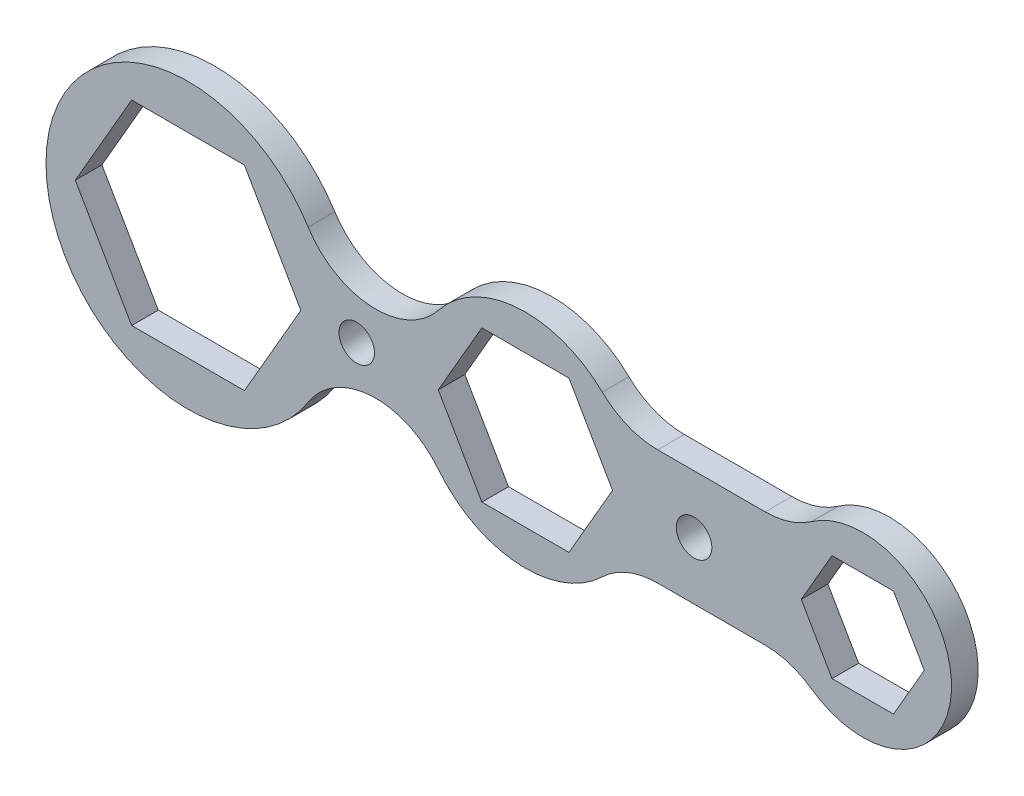
ISO-10303-21;
HEADER;
FILE_DESCRIPTION(('STEP AP214'),'2;1');
FILE_NAME('part.step','',(''),(''),'','','');
FILE_SCHEMA(('AUTOMOTIVE_DESIGN { 1 0 10303 214 1 1 1 1 }'));
ENDSEC;
DATA;
#1=APPLICATION_CONTEXT('core data for automotive mechanical design processes');
#2=APPLICATION_PROTOCOL_DEFINITION('international standard','automotive_design',2000,#1);
#3=PRODUCT_CONTEXT('',#1,'mechanical');
#4=PRODUCT('Part','Part','',(#3));
#5=PRODUCT_RELATED_PRODUCT_CATEGORY('part','',(#4));
#6=PRODUCT_DEFINITION_FORMATION('','',#4);
#7=PRODUCT_DEFINITION_CONTEXT('part definition',#1,'design');
#8=PRODUCT_DEFINITION('design','',#6,#7);
#9=PRODUCT_DEFINITION_SHAPE('','',#8);
#10=(LENGTH_UNIT() NAMED_UNIT(*) SI_UNIT(.MILLI.,.METRE.));
#11=(NAMED_UNIT(*) PLANE_ANGLE_UNIT() SI_UNIT($,.RADIAN.));
#12=(NAMED_UNIT(*) SI_UNIT($,.STERADIAN.) SOLID_ANGLE_UNIT());
#13=UNCERTAINTY_MEASURE_WITH_UNIT(LENGTH_MEASURE(1.E-05),#10,'distance_accuracy_value','');
#14=(GEOMETRIC_REPRESENTATION_CONTEXT(3) GLOBAL_UNCERTAINTY_ASSIGNED_CONTEXT((#13)) GLOBAL_UNIT_ASSIGNED_CONTEXT((#10,
#11,#12)) REPRESENTATION_CONTEXT('',''));
#15=CARTESIAN_POINT('',(0.,0.,0.));
#16=DIRECTION('',(0.,0.,1.));
#17=DIRECTION('',(1.,0.,0.));
#18=AXIS2_PLACEMENT_3D('',#15,#16,#17);
#19=CARTESIAN_POINT('',(76.,0.,6.));
#20=DIRECTION('',(0.,0.,-1.));
#21=DIRECTION('',(-1.,0.,0.));
#22=AXIS2_PLACEMENT_3D('',#19,#20,#21);
#23=CYLINDRICAL_SURFACE('',#22,25.);
#24=CARTESIAN_POINT('',(76.,0.,0.));
#25=DIRECTION('',(0.,0.,1.));
#26=DIRECTION('',(1.,0.,0.));
#27=AXIS2_PLACEMENT_3D('',#24,#25,#26);
#28=CIRCLE('',#27,25.);
#29=CARTESIAN_POINT('',(93.3251911927341,18.0232558139535,0.));
#30=VERTEX_POINT('',#29);
#31=CARTESIAN_POINT('',(56.3970318237454,15.5152711442872,0.));
#32=VERTEX_POINT('',#31);
#33=EDGE_CURVE('E290',#30,#32,#28,.T.);
#34=ORIENTED_EDGE('',*,*,#33,.T.);
#35=DIRECTION('',(0.,0.,-1.));
#36=VECTOR('',#35,1.);
#37=CARTESIAN_POINT('',(56.3970318237454,15.5152711442872,6.));
#38=LINE('',#37,#36);
#39=CARTESIAN_POINT('',(56.3970318237454,15.5152711442872,6.));
#40=VERTEX_POINT('',#39);
#41=EDGE_CURVE('E11',#40,#32,#38,.T.);
#42=ORIENTED_EDGE('',*,*,#41,.F.);
#43=CARTESIAN_POINT('',(76.,0.,6.));
#44=DIRECTION('',(0.,0.,1.));
#45=DIRECTION('',(1.,0.,0.));
#46=AXIS2_PLACEMENT_3D('',#43,#44,#45);
#47=CIRCLE('',#46,25.);
#48=CARTESIAN_POINT('',(93.3251911927341,18.0232558139535,6.));
#49=VERTEX_POINT('',#48);
#50=EDGE_CURVE('E386',#49,#40,#47,.T.);
#51=ORIENTED_EDGE('',*,*,#50,.F.);
#52=DIRECTION('',(0.,0.,-1.));
#53=VECTOR('',#52,1.);
#54=CARTESIAN_POINT('',(93.3251911927341,18.0232558139535,6.));
#55=LINE('',#54,#53);
#56=EDGE_CURVE('E411',#49,#30,#55,.T.);
#57=ORIENTED_EDGE('',*,*,#56,.T.);
#58=EDGE_LOOP('',(#34,#42,#51,#57));
#59=FACE_BOUND('',#58,.T.);
#60=ADVANCED_FACE('F39',(#59),#23,.T.);
#61=CARTESIAN_POINT('',(42.2828947368421,26.6862663681739,6.));
#62=DIRECTION('',(0.,0.,-1.));
#63=DIRECTION('',(-1.,0.,0.));
#64=AXIS2_PLACEMENT_3D('',#61,#62,#63);
#65=CYLINDRICAL_SURFACE('',#64,18.);
#66=CARTESIAN_POINT('',(42.2828947368421,26.6862663681739,0.));
#67=DIRECTION('',(0.,0.,-1.));
#68=DIRECTION('',(1.,0.,0.));
#69=AXIS2_PLACEMENT_3D('',#66,#67,#68);
#70=CIRCLE('',#69,18.);
#71=CARTESIAN_POINT('',(27.0610526315789,17.0792104756313,0.));
#72=VERTEX_POINT('',#71);
#73=EDGE_CURVE('E416',#32,#72,#70,.T.);
#74=ORIENTED_EDGE('',*,*,#73,.T.);
#75=DIRECTION('',(0.,0.,-1.));
#76=VECTOR('',#75,1.);
#77=CARTESIAN_POINT('',(27.0610526315789,17.0792104756313,6.));
#78=LINE('',#77,#76);
#79=CARTESIAN_POINT('',(27.0610526315789,17.0792104756313,6.));
#80=VERTEX_POINT('',#79);
#81=EDGE_CURVE('E46',#80,#72,#78,.T.);
#82=ORIENTED_EDGE('',*,*,#81,.F.);
#83=CARTESIAN_POINT('',(42.2828947368421,26.6862663681739,6.));
#84=DIRECTION('',(0.,0.,-1.));
#85=DIRECTION('',(1.,0.,0.));
#86=AXIS2_PLACEMENT_3D('',#83,#84,#85);
#87=CIRCLE('',#86,18.);
#88=EDGE_CURVE('E395',#40,#80,#87,.T.);
#89=ORIENTED_EDGE('',*,*,#88,.F.);
#90=ORIENTED_EDGE('',*,*,#41,.T.);
#91=EDGE_LOOP('',(#74,#82,#89,#90));
#92=FACE_BOUND('',#91,.T.);
#93=ADVANCED_FACE('F493',(#92),#65,.F.);
#94=CARTESIAN_POINT('',(0.,0.,6.));
#95=DIRECTION('',(0.,0.,-1.));
#96=DIRECTION('',(-1.,0.,0.));
#97=AXIS2_PLACEMENT_3D('',#94,#95,#96);
#98=CYLINDRICAL_SURFACE('',#97,32.);
#99=CARTESIAN_POINT('',(0.,0.,0.));
#100=DIRECTION('',(0.,0.,1.));
#101=DIRECTION('',(1.,0.,0.));
#102=AXIS2_PLACEMENT_3D('',#99,#100,#101);
#103=CIRCLE('',#102,32.);
#104=CARTESIAN_POINT('',(27.0610526315789,-17.0792104756313,0.));
#105=VERTEX_POINT('',#104);
#106=EDGE_CURVE('E419',#72,#105,#103,.T.);
#107=ORIENTED_EDGE('',*,*,#106,.T.);
#108=DIRECTION('',(0.,0.,-1.));
#109=VECTOR('',#108,1.);
#110=CARTESIAN_POINT('',(27.0610526315789,-17.0792104756313,6.));
#111=LINE('',#110,#109);
#112=CARTESIAN_POINT('',(27.0610526315789,-17.0792104756313,6.));
#113=VERTEX_POINT('',#112);
#114=EDGE_CURVE('E464',#113,#105,#111,.T.);
#115=ORIENTED_EDGE('',*,*,#114,.F.);
#116=CARTESIAN_POINT('',(0.,0.,6.));
#117=DIRECTION('',(0.,0.,1.));
#118=DIRECTION('',(1.,0.,0.));
#119=AXIS2_PLACEMENT_3D('',#116,#117,#118);
#120=CIRCLE('',#119,32.);
#121=EDGE_CURVE('E394',#80,#113,#120,.T.);
#122=ORIENTED_EDGE('',*,*,#121,.F.);
#123=ORIENTED_EDGE('',*,*,#81,.T.);
#124=EDGE_LOOP('',(#107,#115,#122,#123));
#125=FACE_BOUND('',#124,.T.);
#126=ADVANCED_FACE('F472',(#125),#98,.T.);
#127=CARTESIAN_POINT('',(42.2828947368421,-26.6862663681739,6.));
#128=DIRECTION('',(0.,0.,-1.));
#129=DIRECTION('',(-1.,0.,0.));
#130=AXIS2_PLACEMENT_3D('',#127,#128,#129);
#131=CYLINDRICAL_SURFACE('',#130,18.);
#132=CARTESIAN_POINT('',(42.2828947368421,-26.6862663681739,0.));
#133=DIRECTION('',(0.,0.,-1.));
#134=DIRECTION('',(1.,0.,0.));
#135=AXIS2_PLACEMENT_3D('',#132,#133,#134);
#136=CIRCLE('',#135,18.);
#137=CARTESIAN_POINT('',(56.3970318237454,-15.5152711442872,0.));
#138=VERTEX_POINT('',#137);
#139=EDGE_CURVE('E425',#105,#138,#136,.T.);
#140=ORIENTED_EDGE('',*,*,#139,.T.);
#141=DIRECTION('',(0.,0.,-1.));
#142=VECTOR('',#141,1.);
#143=CARTESIAN_POINT('',(56.3970318237454,-15.5152711442872,6.));
#144=LINE('',#143,#142);
#145=CARTESIAN_POINT('',(56.3970318237454,-15.5152711442872,6.));
#146=VERTEX_POINT('',#145);
#147=EDGE_CURVE('E465',#146,#138,#144,.T.);
#148=ORIENTED_EDGE('',*,*,#147,.F.);
#149=CARTESIAN_POINT('',(42.2828947368421,-26.6862663681739,6.));
#150=DIRECTION('',(0.,0.,-1.));
#151=DIRECTION('',(1.,0.,0.));
#152=AXIS2_PLACEMENT_3D('',#149,#150,#151);
#153=CIRCLE('',#152,18.);
#154=EDGE_CURVE('E400',#113,#146,#153,.T.);
#155=ORIENTED_EDGE('',*,*,#154,.F.);
#156=ORIENTED_EDGE('',*,*,#114,.T.);
#157=EDGE_LOOP('',(#140,#148,#155,#156));
#158=FACE_BOUND('',#157,.T.);
#159=ADVANCED_FACE('F485',(#158),#131,.F.);
#160=CARTESIAN_POINT('',(76.,0.,6.));
#161=DIRECTION('',(0.,0.,-1.));
#162=DIRECTION('',(-1.,0.,0.));
#163=AXIS2_PLACEMENT_3D('',#160,#161,#162);
#164=CYLINDRICAL_SURFACE('',#163,25.);
#165=CARTESIAN_POINT('',(76.,0.,0.));
#166=DIRECTION('',(0.,0.,1.));
#167=DIRECTION('',(1.,0.,0.));
#168=AXIS2_PLACEMENT_3D('',#165,#166,#167);
#169=CIRCLE('',#168,25.);
#170=CARTESIAN_POINT('',(93.3251911927341,-18.0232558139535,0.));
#171=VERTEX_POINT('',#170);
#172=EDGE_CURVE('E424',#138,#171,#169,.T.);
#173=ORIENTED_EDGE('',*,*,#172,.T.);
#174=DIRECTION('',(0.,0.,-1.));
#175=VECTOR('',#174,1.);
#176=CARTESIAN_POINT('',(93.3251911927341,-18.0232558139535,6.));
#177=LINE('',#176,#175);
#178=CARTESIAN_POINT('',(93.3251911927341,-18.0232558139535,6.));
#179=VERTEX_POINT('',#178);
#180=EDGE_CURVE('E459',#179,#171,#177,.T.);
#181=ORIENTED_EDGE('',*,*,#180,.F.);
#182=CARTESIAN_POINT('',(76.,0.,6.));
#183=DIRECTION('',(0.,0.,1.));
#184=DIRECTION('',(1.,0.,0.));
#185=AXIS2_PLACEMENT_3D('',#182,#183,#184);
#186=CIRCLE('',#185,25.);
#187=EDGE_CURVE('E399',#146,#179,#186,.T.);
#188=ORIENTED_EDGE('',*,*,#187,.F.);
#189=ORIENTED_EDGE('',*,*,#147,.T.);
#190=EDGE_LOOP('',(#173,#181,#188,#189));
#191=FACE_BOUND('',#190,.T.);
#192=ADVANCED_FACE('F486',(#191),#164,.T.);
#193=CARTESIAN_POINT('',(105.799328851503,-31.,6.));
#194=DIRECTION('',(0.,0.,-1.));
#195=DIRECTION('',(-1.,0.,0.));
#196=AXIS2_PLACEMENT_3D('',#193,#194,#195);
#197=CYLINDRICAL_SURFACE('',#196,18.);
#198=CARTESIAN_POINT('',(105.799328851503,-31.,0.));
#199=DIRECTION('',(0.,0.,-1.));
#200=DIRECTION('',(1.,0.,0.));
#201=AXIS2_PLACEMENT_3D('',#198,#199,#200);
#202=CIRCLE('',#201,18.);
#203=CARTESIAN_POINT('',(105.799328851503,-13.,0.));
#204=VERTEX_POINT('',#203);
#205=EDGE_CURVE('E426',#171,#204,#202,.T.);
#206=ORIENTED_EDGE('',*,*,#205,.T.);
#207=DIRECTION('',(0.,0.,-1.));
#208=VECTOR('',#207,1.);
#209=CARTESIAN_POINT('',(105.799328851503,-13.,6.));
#210=LINE('',#209,#208);
#211=CARTESIAN_POINT('',(105.799328851503,-13.,6.));
#212=VERTEX_POINT('',#211);
#213=EDGE_CURVE('E457',#212,#204,#210,.T.);
#214=ORIENTED_EDGE('',*,*,#213,.F.);
#215=CARTESIAN_POINT('',(105.799328851503,-31.,6.));
#216=DIRECTION('',(0.,0.,-1.));
#217=DIRECTION('',(1.,0.,0.));
#218=AXIS2_PLACEMENT_3D('',#215,#216,#217);
#219=CIRCLE('',#218,18.);
#220=EDGE_CURVE('E402',#179,#212,#219,.T.);
#221=ORIENTED_EDGE('',*,*,#220,.F.);
#222=ORIENTED_EDGE('',*,*,#180,.T.);
#223=EDGE_LOOP('',(#206,#214,#221,#222));
#224=FACE_BOUND('',#223,.T.);
#225=ADVANCED_FACE('F527',(#224),#197,.F.);
#226=CARTESIAN_POINT('',(105.799328851503,-13.,6.));
#227=DIRECTION('',(0.,1.,0.));
#228=DIRECTION('',(-1.,0.,0.));
#229=AXIS2_PLACEMENT_3D('',#226,#227,#228);
#230=PLANE('',#229);
#231=DIRECTION('',(1.,0.,0.));
#232=VECTOR('',#231,1.);
#233=CARTESIAN_POINT('',(105.799328851503,-13.,0.));
#234=LINE('',#233,#232);
#235=CARTESIAN_POINT('',(130.022739024164,-13.,0.));
#236=VERTEX_POINT('',#235);
#237=EDGE_CURVE('E428',#204,#236,#234,.T.);
#238=ORIENTED_EDGE('',*,*,#237,.T.);
#239=DIRECTION('',(0.,0.,-1.));
#240=VECTOR('',#239,1.);
#241=CARTESIAN_POINT('',(130.022739024164,-13.,6.));
#242=LINE('',#241,#240);
#243=CARTESIAN_POINT('',(130.022739024164,-13.,6.));
#244=VERTEX_POINT('',#243);
#245=EDGE_CURVE('E453',#244,#236,#242,.T.);
#246=ORIENTED_EDGE('',*,*,#245,.F.);
#247=DIRECTION('',(1.,0.,0.));
#248=VECTOR('',#247,1.);
#249=CARTESIAN_POINT('',(105.799328851503,-13.,6.));
#250=LINE('',#249,#248);
#251=EDGE_CURVE('E401',#212,#244,#250,.T.);
#252=ORIENTED_EDGE('',*,*,#251,.F.);
#253=ORIENTED_EDGE('',*,*,#213,.T.);
#254=EDGE_LOOP('',(#238,#246,#252,#253));
#255=FACE_BOUND('',#254,.T.);
#256=ADVANCED_FACE('F521',(#255),#230,.F.);
#257=CARTESIAN_POINT('',(130.022739024164,-31.,6.));
#258=DIRECTION('',(0.,0.,-1.));
#259=DIRECTION('',(-1.,0.,0.));
#260=AXIS2_PLACEMENT_3D('',#257,#258,#259);
#261=CYLINDRICAL_SURFACE('',#260,18.);
#262=CARTESIAN_POINT('',(130.022739024164,-31.,0.));
#263=DIRECTION('',(0.,0.,-1.));
#264=DIRECTION('',(1.,0.,0.));
#265=AXIS2_PLACEMENT_3D('',#262,#263,#264);
#266=CIRCLE('',#265,18.);
#267=CARTESIAN_POINT('',(140.433020539034,-16.3157894736842,0.));
#268=VERTEX_POINT('',#267);
#269=EDGE_CURVE('E429',#236,#268,#266,.T.);
#270=ORIENTED_EDGE('',*,*,#269,.T.);
#271=DIRECTION('',(0.,0.,-1.));
#272=VECTOR('',#271,1.);
#273=CARTESIAN_POINT('',(140.433020539034,-16.3157894736842,6.));
#274=LINE('',#273,#272);
#275=CARTESIAN_POINT('',(140.433020539034,-16.3157894736842,6.));
#276=VERTEX_POINT('',#275);
#277=EDGE_CURVE('E449',#276,#268,#274,.T.);
#278=ORIENTED_EDGE('',*,*,#277,.F.);
#279=CARTESIAN_POINT('',(130.022739024164,-31.,6.));
#280=DIRECTION('',(0.,0.,-1.));
#281=DIRECTION('',(1.,0.,0.));
#282=AXIS2_PLACEMENT_3D('',#279,#280,#281);
#283=CIRCLE('',#282,18.);
#284=EDGE_CURVE('E403',#244,#276,#283,.T.);
#285=ORIENTED_EDGE('',*,*,#284,.F.);
#286=ORIENTED_EDGE('',*,*,#245,.T.);
#287=EDGE_LOOP('',(#270,#278,#285,#286));
#288=FACE_BOUND('',#287,.T.);
#289=ADVANCED_FACE('F522',(#288),#261,.F.);
#290=CARTESIAN_POINT('',(152.,0.,6.));
#291=DIRECTION('',(0.,0.,-1.));
#292=DIRECTION('',(-1.,0.,0.));
#293=AXIS2_PLACEMENT_3D('',#290,#291,#292);
#294=CYLINDRICAL_SURFACE('',#293,20.);
#295=CARTESIAN_POINT('',(152.,0.,0.));
#296=DIRECTION('',(0.,0.,1.));
#297=DIRECTION('',(1.,0.,0.));
#298=AXIS2_PLACEMENT_3D('',#295,#296,#297);
#299=CIRCLE('',#298,20.);
#300=CARTESIAN_POINT('',(140.433020539034,16.3157894736842,0.));
#301=VERTEX_POINT('',#300);
#302=EDGE_CURVE('E435',#268,#301,#299,.T.);
#303=ORIENTED_EDGE('',*,*,#302,.T.);
#304=DIRECTION('',(0.,0.,-1.));
#305=VECTOR('',#304,1.);
#306=CARTESIAN_POINT('',(140.433020539034,16.3157894736842,6.));
#307=LINE('',#306,#305);
#308=CARTESIAN_POINT('',(140.433020539034,16.3157894736842,6.));
#309=VERTEX_POINT('',#308);
#310=EDGE_CURVE('E450',#309,#301,#307,.T.);
#311=ORIENTED_EDGE('',*,*,#310,.F.);
#312=CARTESIAN_POINT('',(152.,0.,6.));
#313=DIRECTION('',(0.,0.,1.));
#314=DIRECTION('',(1.,0.,0.));
#315=AXIS2_PLACEMENT_3D('',#312,#313,#314);
#316=CIRCLE('',#315,20.);
#317=EDGE_CURVE('E410',#276,#309,#316,.T.);
#318=ORIENTED_EDGE('',*,*,#317,.F.);
#319=ORIENTED_EDGE('',*,*,#277,.T.);
#320=EDGE_LOOP('',(#303,#311,#318,#319));
#321=FACE_BOUND('',#320,.T.);
#322=ADVANCED_FACE('F516',(#321),#294,.T.);
#323=CARTESIAN_POINT('',(130.022739024164,31.,6.));
#324=DIRECTION('',(0.,0.,-1.));
#325=DIRECTION('',(-1.,0.,0.));
#326=AXIS2_PLACEMENT_3D('',#323,#324,#325);
#327=CYLINDRICAL_SURFACE('',#326,18.);
#328=CARTESIAN_POINT('',(130.022739024164,31.,0.));
#329=DIRECTION('',(0.,0.,-1.));
#330=DIRECTION('',(1.,0.,0.));
#331=AXIS2_PLACEMENT_3D('',#328,#329,#330);
#332=CIRCLE('',#331,18.);
#333=CARTESIAN_POINT('',(130.022739024164,13.,0.));
#334=VERTEX_POINT('',#333);
#335=EDGE_CURVE('E432',#301,#334,#332,.T.);
#336=ORIENTED_EDGE('',*,*,#335,.T.);
#337=DIRECTION('',(0.,0.,-1.));
#338=VECTOR('',#337,1.);
#339=CARTESIAN_POINT('',(130.022739024164,13.,6.));
#340=LINE('',#339,#338);
#341=CARTESIAN_POINT('',(130.022739024164,13.,6.));
#342=VERTEX_POINT('',#341);
#343=EDGE_CURVE('E441',#342,#334,#340,.T.);
#344=ORIENTED_EDGE('',*,*,#343,.F.);
#345=CARTESIAN_POINT('',(130.022739024164,31.,6.));
#346=DIRECTION('',(0.,0.,-1.));
#347=DIRECTION('',(1.,0.,0.));
#348=AXIS2_PLACEMENT_3D('',#345,#346,#347);
#349=CIRCLE('',#348,18.);
#350=EDGE_CURVE('E408',#309,#342,#349,.T.);
#351=ORIENTED_EDGE('',*,*,#350,.F.);
#352=ORIENTED_EDGE('',*,*,#310,.T.);
#353=EDGE_LOOP('',(#336,#344,#351,#352));
#354=FACE_BOUND('',#353,.T.);
#355=ADVANCED_FACE('F506',(#354),#327,.F.);
#356=CARTESIAN_POINT('',(105.799328851503,13.,6.));
#357=DIRECTION('',(0.,-1.,0.));
#358=DIRECTION('',(1.,0.,0.));
#359=AXIS2_PLACEMENT_3D('',#356,#357,#358);
#360=PLANE('',#359);
#361=DIRECTION('',(-1.,0.,0.));
#362=VECTOR('',#361,1.);
#363=CARTESIAN_POINT('',(105.799328851503,13.,0.));
#364=LINE('',#363,#362);
#365=CARTESIAN_POINT('',(105.799328851503,13.,0.));
#366=VERTEX_POINT('',#365);
#367=EDGE_CURVE('E436',#334,#366,#364,.T.);
#368=ORIENTED_EDGE('',*,*,#367,.T.);
#369=DIRECTION('',(0.,0.,-1.));
#370=VECTOR('',#369,1.);
#371=CARTESIAN_POINT('',(105.799328851503,13.,6.));
#372=LINE('',#371,#370);
#373=CARTESIAN_POINT('',(105.799328851503,13.,6.));
#374=VERTEX_POINT('',#373);
#375=EDGE_CURVE('E442',#374,#366,#372,.T.);
#376=ORIENTED_EDGE('',*,*,#375,.F.);
#377=DIRECTION('',(-1.,0.,0.));
#378=VECTOR('',#377,1.);
#379=CARTESIAN_POINT('',(105.799328851503,13.,6.));
#380=LINE('',#379,#378);
#381=EDGE_CURVE('E412',#342,#374,#380,.T.);
#382=ORIENTED_EDGE('',*,*,#381,.F.);
#383=ORIENTED_EDGE('',*,*,#343,.T.);
#384=EDGE_LOOP('',(#368,#376,#382,#383));
#385=FACE_BOUND('',#384,.T.);
#386=ADVANCED_FACE('F507',(#385),#360,.F.);
#387=CARTESIAN_POINT('',(105.799328851503,31.,6.));
#388=DIRECTION('',(0.,0.,-1.));
#389=DIRECTION('',(-1.,0.,0.));
#390=AXIS2_PLACEMENT_3D('',#387,#388,#389);
#391=CYLINDRICAL_SURFACE('',#390,18.);
#392=CARTESIAN_POINT('',(105.799328851503,31.,0.));
#393=DIRECTION('',(0.,0.,-1.));
#394=DIRECTION('',(1.,0.,0.));
#395=AXIS2_PLACEMENT_3D('',#392,#393,#394);
#396=CIRCLE('',#395,18.);
#397=EDGE_CURVE('E392',#366,#30,#396,.T.);
#398=ORIENTED_EDGE('',*,*,#397,.T.);
#399=ORIENTED_EDGE('',*,*,#56,.F.);
#400=CARTESIAN_POINT('',(105.799328851503,31.,6.));
#401=DIRECTION('',(0.,0.,-1.));
#402=DIRECTION('',(1.,0.,0.));
#403=AXIS2_PLACEMENT_3D('',#400,#401,#402);
#404=CIRCLE('',#403,18.);
#405=EDGE_CURVE('E413',#374,#49,#404,.T.);
#406=ORIENTED_EDGE('',*,*,#405,.F.);
#407=ORIENTED_EDGE('',*,*,#375,.T.);
#408=EDGE_LOOP('',(#398,#399,#406,#407));
#409=FACE_BOUND('',#408,.T.);
#410=ADVANCED_FACE('F501',(#409),#391,.F.);
#411=CARTESIAN_POINT('',(76.,0.,6.));
#412=DIRECTION('',(0.,0.,1.));
#413=DIRECTION('',(1.,0.,0.));
#414=AXIS2_PLACEMENT_3D('',#411,#412,#413);
#415=PLANE('',#414);
#416=CARTESIAN_POINT('',(38.,0.,6.));
#417=DIRECTION('',(0.,0.,1.));
#418=DIRECTION('',(1.,0.,0.));
#419=AXIS2_PLACEMENT_3D('',#416,#417,#418);
#420=CIRCLE('',#419,4.00000000000001);
#421=CARTESIAN_POINT('',(42.,0.,6.));
#422=VERTEX_POINT('',#421);
#423=EDGE_CURVE('E830',#422,#422,#420,.T.);
#424=ORIENTED_EDGE('',*,*,#423,.F.);
#425=EDGE_LOOP('',(#424));
#426=FACE_BOUND('',#425,.T.);
#427=CARTESIAN_POINT('',(114.,0.,6.));
#428=DIRECTION('',(0.,0.,1.));
#429=DIRECTION('',(1.,0.,0.));
#430=AXIS2_PLACEMENT_3D('',#427,#428,#429);
#431=CIRCLE('',#430,4.00000000000001);
#432=CARTESIAN_POINT('',(118.,0.,6.));
#433=VERTEX_POINT('',#432);
#434=EDGE_CURVE('E263',#433,#433,#431,.T.);
#435=ORIENTED_EDGE('',*,*,#434,.F.);
#436=EDGE_LOOP('',(#435));
#437=FACE_BOUND('',#436,.T.);
#438=DIRECTION('',(0.5,0.866025403784438,0.));
#439=VECTOR('',#438,1.);
#440=CARTESIAN_POINT('',(12.7017059221718,-22.,6.));
#441=LINE('',#440,#439);
#442=CARTESIAN_POINT('',(12.7017059221718,-22.,6.));
#443=VERTEX_POINT('',#442);
#444=CARTESIAN_POINT('',(25.4034118443435,0.,6.));
#445=VERTEX_POINT('',#444);
#446=EDGE_CURVE('E52',#443,#445,#441,.T.);
#447=ORIENTED_EDGE('',*,*,#446,.F.);
#448=DIRECTION('',(1.,0.,0.));
#449=VECTOR('',#448,1.);
#450=CARTESIAN_POINT('',(-12.7017059221718,-22.,6.));
#451=LINE('',#450,#449);
#452=CARTESIAN_POINT('',(-12.7017059221718,-22.,6.));
#453=VERTEX_POINT('',#452);
#454=EDGE_CURVE('E260',#453,#443,#451,.T.);
#455=ORIENTED_EDGE('',*,*,#454,.F.);
#456=DIRECTION('',(0.5,-0.866025403784439,0.));
#457=VECTOR('',#456,1.);
#458=CARTESIAN_POINT('',(-25.4034118443435,0.,6.));
#459=LINE('',#458,#457);
#460=CARTESIAN_POINT('',(-25.4034118443435,0.,6.));
#461=VERTEX_POINT('',#460);
#462=EDGE_CURVE('E257',#461,#453,#459,.T.);
#463=ORIENTED_EDGE('',*,*,#462,.F.);
#464=DIRECTION('',(-0.5,-0.866025403784438,0.));
#465=VECTOR('',#464,1.);
#466=CARTESIAN_POINT('',(-12.7017059221718,22.,6.));
#467=LINE('',#466,#465);
#468=CARTESIAN_POINT('',(-12.7017059221718,22.,6.));
#469=VERTEX_POINT('',#468);
#470=EDGE_CURVE('E278',#469,#461,#467,.T.);
#471=ORIENTED_EDGE('',*,*,#470,.F.);
#472=DIRECTION('',(-1.,0.,0.));
#473=VECTOR('',#472,1.);
#474=CARTESIAN_POINT('',(12.7017059221718,22.,6.));
#475=LINE('',#474,#473);
#476=CARTESIAN_POINT('',(12.7017059221718,22.,6.));
#477=VERTEX_POINT('',#476);
#478=EDGE_CURVE('E280',#477,#469,#475,.T.);
#479=ORIENTED_EDGE('',*,*,#478,.F.);
#480=DIRECTION('',(-0.5,0.866025403784439,0.));
#481=VECTOR('',#480,1.);
#482=CARTESIAN_POINT('',(25.4034118443435,0.,6.));
#483=LINE('',#482,#481);
#484=EDGE_CURVE('E273',#445,#477,#483,.T.);
#485=ORIENTED_EDGE('',*,*,#484,.F.);
#486=EDGE_LOOP('',(#447,#455,#463,#471,#479,#485));
#487=FACE_BOUND('',#486,.T.);
#488=DIRECTION('',(0.5,0.866025403784439,0.));
#489=VECTOR('',#488,1.);
#490=CARTESIAN_POINT('',(85.8149545762236,-17.,6.));
#491=LINE('',#490,#489);
#492=CARTESIAN_POINT('',(85.8149545762236,-17.,6.));
#493=VERTEX_POINT('',#492);
#494=CARTESIAN_POINT('',(95.6299091524473,0.,6.));
#495=VERTEX_POINT('',#494);
#496=EDGE_CURVE('E61',#493,#495,#491,.T.);
#497=ORIENTED_EDGE('',*,*,#496,.F.);
#498=DIRECTION('',(1.,0.,0.));
#499=VECTOR('',#498,1.);
#500=CARTESIAN_POINT('',(66.1850454237763,-17.,6.));
#501=LINE('',#500,#499);
#502=CARTESIAN_POINT('',(66.1850454237763,-17.,6.));
#503=VERTEX_POINT('',#502);
#504=EDGE_CURVE('E298',#503,#493,#501,.T.);
#505=ORIENTED_EDGE('',*,*,#504,.F.);
#506=DIRECTION('',(0.5,-0.866025403784439,0.));
#507=VECTOR('',#506,1.);
#508=CARTESIAN_POINT('',(56.3700908475527,0.,6.));
#509=LINE('',#508,#507);
#510=CARTESIAN_POINT('',(56.3700908475527,0.,6.));
#511=VERTEX_POINT('',#510);
#512=EDGE_CURVE('E326',#511,#503,#509,.T.);
#513=ORIENTED_EDGE('',*,*,#512,.F.);
#514=DIRECTION('',(-0.5,-0.866025403784439,0.));
#515=VECTOR('',#514,1.);
#516=CARTESIAN_POINT('',(66.1850454237763,17.,6.));
#517=LINE('',#516,#515);
#518=CARTESIAN_POINT('',(66.1850454237763,17.,6.));
#519=VERTEX_POINT('',#518);
#520=EDGE_CURVE('E323',#519,#511,#517,.T.);
#521=ORIENTED_EDGE('',*,*,#520,.F.);
#522=DIRECTION('',(-1.,0.,0.));
#523=VECTOR('',#522,1.);
#524=CARTESIAN_POINT('',(85.8149545762236,17.,6.));
#525=LINE('',#524,#523);
#526=CARTESIAN_POINT('',(85.8149545762236,17.,6.));
#527=VERTEX_POINT('',#526);
#528=EDGE_CURVE('E319',#527,#519,#525,.T.);
#529=ORIENTED_EDGE('',*,*,#528,.F.);
#530=DIRECTION('',(-0.5,0.866025403784438,0.));
#531=VECTOR('',#530,1.);
#532=CARTESIAN_POINT('',(95.6299091524473,0.,6.));
#533=LINE('',#532,#531);
#534=EDGE_CURVE('E316',#495,#527,#533,.T.);
#535=ORIENTED_EDGE('',*,*,#534,.F.);
#536=EDGE_LOOP('',(#497,#505,#513,#521,#529,#535));
#537=FACE_BOUND('',#536,.T.);
#538=DIRECTION('',(0.499999999999999,0.866025403784439,0.));
#539=VECTOR('',#538,1.);
#540=CARTESIAN_POINT('',(158.928203230276,-12.,6.));
#541=LINE('',#540,#539);
#542=CARTESIAN_POINT('',(158.928203230276,-12.,6.));
#543=VERTEX_POINT('',#542);
#544=CARTESIAN_POINT('',(165.856406460551,0.,6.));
#545=VERTEX_POINT('',#544);
#546=EDGE_CURVE('E363',#543,#545,#541,.T.);
#547=ORIENTED_EDGE('',*,*,#546,.F.);
#548=DIRECTION('',(1.,0.,0.));
#549=VECTOR('',#548,1.);
#550=CARTESIAN_POINT('',(145.071796769724,-12.,6.));
#551=LINE('',#550,#549);
#552=CARTESIAN_POINT('',(145.071796769724,-12.,6.));
#553=VERTEX_POINT('',#552);
#554=EDGE_CURVE('E341',#553,#543,#551,.T.);
#555=ORIENTED_EDGE('',*,*,#554,.F.);
#556=DIRECTION('',(0.500000000000001,-0.866025403784438,0.));
#557=VECTOR('',#556,1.);
#558=CARTESIAN_POINT('',(138.143593539449,0.,6.));
#559=LINE('',#558,#557);
#560=CARTESIAN_POINT('',(138.143593539449,0.,6.));
#561=VERTEX_POINT('',#560);
#562=EDGE_CURVE('E373',#561,#553,#559,.T.);
#563=ORIENTED_EDGE('',*,*,#562,.F.);
#564=DIRECTION('',(-0.500000000000001,-0.866025403784438,0.));
#565=VECTOR('',#564,1.);
#566=CARTESIAN_POINT('',(145.071796769725,12.,6.));
#567=LINE('',#566,#565);
#568=CARTESIAN_POINT('',(145.071796769725,12.,6.));
#569=VERTEX_POINT('',#568);
#570=EDGE_CURVE('E367',#569,#561,#567,.T.);
#571=ORIENTED_EDGE('',*,*,#570,.F.);
#572=DIRECTION('',(-1.,0.,0.));
#573=VECTOR('',#572,1.);
#574=CARTESIAN_POINT('',(158.928203230275,12.,6.));
#575=LINE('',#574,#573);
#576=CARTESIAN_POINT('',(158.928203230275,12.,6.));
#577=VERTEX_POINT('',#576);
#578=EDGE_CURVE('E370',#577,#569,#575,.T.);
#579=ORIENTED_EDGE('',*,*,#578,.F.);
#580=DIRECTION('',(-0.500000000000001,0.866025403784438,0.));
#581=VECTOR('',#580,1.);
#582=CARTESIAN_POINT('',(165.856406460551,0.,6.));
#583=LINE('',#582,#581);
#584=EDGE_CURVE('E361',#545,#577,#583,.T.);
#585=ORIENTED_EDGE('',*,*,#584,.F.);
#586=EDGE_LOOP('',(#547,#555,#563,#571,#579,#585));
#587=FACE_BOUND('',#586,.T.);
#588=ORIENTED_EDGE('',*,*,#50,.T.);
#589=ORIENTED_EDGE('',*,*,#88,.T.);
#590=ORIENTED_EDGE('',*,*,#121,.T.);
#591=ORIENTED_EDGE('',*,*,#154,.T.);
#592=ORIENTED_EDGE('',*,*,#187,.T.);
#593=ORIENTED_EDGE('',*,*,#220,.T.);
#594=ORIENTED_EDGE('',*,*,#251,.T.);
#595=ORIENTED_EDGE('',*,*,#284,.T.);
#596=ORIENTED_EDGE('',*,*,#317,.T.);
#597=ORIENTED_EDGE('',*,*,#350,.T.);
#598=ORIENTED_EDGE('',*,*,#381,.T.);
#599=ORIENTED_EDGE('',*,*,#405,.T.);
#600=EDGE_LOOP('',(#588,#589,#590,#591,#592,#593,#594,#595,#596,#597,#598,#599));
#601=FACE_BOUND('',#600,.T.);
#602=ADVANCED_FACE('F489',(#426,#437,#487,#537,#587,#601),#415,.T.);
#603=CARTESIAN_POINT('',(76.,0.,0.));
#604=DIRECTION('',(0.,0.,1.));
#605=DIRECTION('',(1.,0.,0.));
#606=AXIS2_PLACEMENT_3D('',#603,#604,#605);
#607=PLANE('',#606);
#608=CARTESIAN_POINT('',(38.,0.,0.));
#609=DIRECTION('',(0.,0.,1.));
#610=DIRECTION('',(1.,0.,0.));
#611=AXIS2_PLACEMENT_3D('',#608,#609,#610);
#612=CIRCLE('',#611,4.00000000000001);
#613=CARTESIAN_POINT('',(42.,0.,0.));
#614=VERTEX_POINT('',#613);
#615=EDGE_CURVE('E365',#614,#614,#612,.T.);
#616=ORIENTED_EDGE('',*,*,#615,.T.);
#617=EDGE_LOOP('',(#616));
#618=FACE_BOUND('',#617,.T.);
#619=CARTESIAN_POINT('',(114.,0.,0.));
#620=DIRECTION('',(0.,0.,1.));
#621=DIRECTION('',(1.,0.,0.));
#622=AXIS2_PLACEMENT_3D('',#619,#620,#621);
#623=CIRCLE('',#622,4.00000000000001);
#624=CARTESIAN_POINT('',(118.,0.,0.));
#625=VERTEX_POINT('',#624);
#626=EDGE_CURVE('E829',#625,#625,#623,.T.);
#627=ORIENTED_EDGE('',*,*,#626,.T.);
#628=EDGE_LOOP('',(#627));
#629=FACE_BOUND('',#628,.T.);
#630=DIRECTION('',(1.,0.,0.));
#631=VECTOR('',#630,1.);
#632=CARTESIAN_POINT('',(-12.7017059221718,-22.,0.));
#633=LINE('',#632,#631);
#634=CARTESIAN_POINT('',(-12.7017059221718,-22.,0.));
#635=VERTEX_POINT('',#634);
#636=CARTESIAN_POINT('',(12.7017059221718,-22.,0.));
#637=VERTEX_POINT('',#636);
#638=EDGE_CURVE('E242',#635,#637,#633,.T.);
#639=ORIENTED_EDGE('',*,*,#638,.T.);
#640=DIRECTION('',(0.5,0.866025403784438,0.));
#641=VECTOR('',#640,1.);
#642=CARTESIAN_POINT('',(12.7017059221718,-22.,0.));
#643=LINE('',#642,#641);
#644=CARTESIAN_POINT('',(25.4034118443435,0.,0.));
#645=VERTEX_POINT('',#644);
#646=EDGE_CURVE('E240',#637,#645,#643,.T.);
#647=ORIENTED_EDGE('',*,*,#646,.T.);
#648=DIRECTION('',(-0.5,0.866025403784439,0.));
#649=VECTOR('',#648,1.);
#650=CARTESIAN_POINT('',(25.4034118443435,0.,0.));
#651=LINE('',#650,#649);
#652=CARTESIAN_POINT('',(12.7017059221718,22.,0.));
#653=VERTEX_POINT('',#652);
#654=EDGE_CURVE('E250',#645,#653,#651,.T.);
#655=ORIENTED_EDGE('',*,*,#654,.T.);
#656=DIRECTION('',(-1.,0.,0.));
#657=VECTOR('',#656,1.);
#658=CARTESIAN_POINT('',(12.7017059221718,22.,0.));
#659=LINE('',#658,#657);
#660=CARTESIAN_POINT('',(-12.7017059221718,22.,0.));
#661=VERTEX_POINT('',#660);
#662=EDGE_CURVE('E253',#653,#661,#659,.T.);
#663=ORIENTED_EDGE('',*,*,#662,.T.);
#664=DIRECTION('',(-0.5,-0.866025403784438,0.));
#665=VECTOR('',#664,1.);
#666=CARTESIAN_POINT('',(-12.7017059221718,22.,0.));
#667=LINE('',#666,#665);
#668=CARTESIAN_POINT('',(-25.4034118443435,0.,0.));
#669=VERTEX_POINT('',#668);
#670=EDGE_CURVE('E270',#661,#669,#667,.T.);
#671=ORIENTED_EDGE('',*,*,#670,.T.);
#672=DIRECTION('',(0.5,-0.866025403784439,0.));
#673=VECTOR('',#672,1.);
#674=CARTESIAN_POINT('',(-25.4034118443435,0.,0.));
#675=LINE('',#674,#673);
#676=EDGE_CURVE('E269',#669,#635,#675,.T.);
#677=ORIENTED_EDGE('',*,*,#676,.T.);
#678=EDGE_LOOP('',(#639,#647,#655,#663,#671,#677));
#679=FACE_BOUND('',#678,.T.);
#680=DIRECTION('',(1.,0.,0.));
#681=VECTOR('',#680,1.);
#682=CARTESIAN_POINT('',(66.1850454237763,-17.,0.));
#683=LINE('',#682,#681);
#684=CARTESIAN_POINT('',(66.1850454237763,-17.,0.));
#685=VERTEX_POINT('',#684);
#686=CARTESIAN_POINT('',(85.8149545762236,-17.,0.));
#687=VERTEX_POINT('',#686);
#688=EDGE_CURVE('E313',#685,#687,#683,.T.);
#689=ORIENTED_EDGE('',*,*,#688,.T.);
#690=DIRECTION('',(0.5,0.866025403784439,0.));
#691=VECTOR('',#690,1.);
#692=CARTESIAN_POINT('',(85.8149545762236,-17.,0.));
#693=LINE('',#692,#691);
#694=CARTESIAN_POINT('',(95.6299091524473,0.,0.));
#695=VERTEX_POINT('',#694);
#696=EDGE_CURVE('E293',#687,#695,#693,.T.);
#697=ORIENTED_EDGE('',*,*,#696,.T.);
#698=DIRECTION('',(-0.5,0.866025403784438,0.));
#699=VECTOR('',#698,1.);
#700=CARTESIAN_POINT('',(95.6299091524473,0.,0.));
#701=LINE('',#700,#699);
#702=CARTESIAN_POINT('',(85.8149545762236,17.,0.));
#703=VERTEX_POINT('',#702);
#704=EDGE_CURVE('E297',#695,#703,#701,.T.);
#705=ORIENTED_EDGE('',*,*,#704,.T.);
#706=DIRECTION('',(-1.,0.,0.));
#707=VECTOR('',#706,1.);
#708=CARTESIAN_POINT('',(85.8149545762236,17.,0.));
#709=LINE('',#708,#707);
#710=CARTESIAN_POINT('',(66.1850454237763,17.,0.));
#711=VERTEX_POINT('',#710);
#712=EDGE_CURVE('E305',#703,#711,#709,.T.);
#713=ORIENTED_EDGE('',*,*,#712,.T.);
#714=DIRECTION('',(-0.5,-0.866025403784439,0.));
#715=VECTOR('',#714,1.);
#716=CARTESIAN_POINT('',(66.1850454237763,17.,0.));
#717=LINE('',#716,#715);
#718=CARTESIAN_POINT('',(56.3700908475527,0.,0.));
#719=VERTEX_POINT('',#718);
#720=EDGE_CURVE('E301',#711,#719,#717,.T.);
#721=ORIENTED_EDGE('',*,*,#720,.T.);
#722=DIRECTION('',(0.5,-0.866025403784439,0.));
#723=VECTOR('',#722,1.);
#724=CARTESIAN_POINT('',(56.3700908475527,0.,0.));
#725=LINE('',#724,#723);
#726=EDGE_CURVE('E306',#719,#685,#725,.T.);
#727=ORIENTED_EDGE('',*,*,#726,.T.);
#728=EDGE_LOOP('',(#689,#697,#705,#713,#721,#727));
#729=FACE_BOUND('',#728,.T.);
#730=DIRECTION('',(1.,0.,0.));
#731=VECTOR('',#730,1.);
#732=CARTESIAN_POINT('',(145.071796769724,-12.,0.));
#733=LINE('',#732,#731);
#734=CARTESIAN_POINT('',(145.071796769724,-12.,0.));
#735=VERTEX_POINT('',#734);
#736=CARTESIAN_POINT('',(158.928203230276,-12.,0.));
#737=VERTEX_POINT('',#736);
#738=EDGE_CURVE('E360',#735,#737,#733,.T.);
#739=ORIENTED_EDGE('',*,*,#738,.T.);
#740=DIRECTION('',(0.499999999999999,0.866025403784439,0.));
#741=VECTOR('',#740,1.);
#742=CARTESIAN_POINT('',(158.928203230276,-12.,0.));
#743=LINE('',#742,#741);
#744=CARTESIAN_POINT('',(165.856406460551,0.,0.));
#745=VERTEX_POINT('',#744);
#746=EDGE_CURVE('E342',#737,#745,#743,.T.);
#747=ORIENTED_EDGE('',*,*,#746,.T.);
#748=DIRECTION('',(-0.500000000000001,0.866025403784438,0.));
#749=VECTOR('',#748,1.);
#750=CARTESIAN_POINT('',(165.856406460551,0.,0.));
#751=LINE('',#750,#749);
#752=CARTESIAN_POINT('',(158.928203230275,12.,0.));
#753=VERTEX_POINT('',#752);
#754=EDGE_CURVE('E344',#745,#753,#751,.T.);
#755=ORIENTED_EDGE('',*,*,#754,.T.);
#756=DIRECTION('',(-1.,0.,0.));
#757=VECTOR('',#756,1.);
#758=CARTESIAN_POINT('',(158.928203230275,12.,0.));
#759=LINE('',#758,#757);
#760=CARTESIAN_POINT('',(145.071796769725,12.,0.));
#761=VERTEX_POINT('',#760);
#762=EDGE_CURVE('E346',#753,#761,#759,.T.);
#763=ORIENTED_EDGE('',*,*,#762,.T.);
#764=DIRECTION('',(-0.500000000000001,-0.866025403784438,0.));
#765=VECTOR('',#764,1.);
#766=CARTESIAN_POINT('',(145.071796769725,12.,0.));
#767=LINE('',#766,#765);
#768=CARTESIAN_POINT('',(138.143593539449,0.,0.));
#769=VERTEX_POINT('',#768);
#770=EDGE_CURVE('E351',#761,#769,#767,.T.);
#771=ORIENTED_EDGE('',*,*,#770,.T.);
#772=DIRECTION('',(0.500000000000001,-0.866025403784438,0.));
#773=VECTOR('',#772,1.);
#774=CARTESIAN_POINT('',(138.143593539449,0.,0.));
#775=LINE('',#774,#773);
#776=EDGE_CURVE('E353',#769,#735,#775,.T.);
#777=ORIENTED_EDGE('',*,*,#776,.T.);
#778=EDGE_LOOP('',(#739,#747,#755,#763,#771,#777));
#779=FACE_BOUND('',#778,.T.);
#780=ORIENTED_EDGE('',*,*,#33,.F.);
#781=ORIENTED_EDGE('',*,*,#397,.F.);
#782=ORIENTED_EDGE('',*,*,#367,.F.);
#783=ORIENTED_EDGE('',*,*,#335,.F.);
#784=ORIENTED_EDGE('',*,*,#302,.F.);
#785=ORIENTED_EDGE('',*,*,#269,.F.);
#786=ORIENTED_EDGE('',*,*,#237,.F.);
#787=ORIENTED_EDGE('',*,*,#205,.F.);
#788=ORIENTED_EDGE('',*,*,#172,.F.);
#789=ORIENTED_EDGE('',*,*,#139,.F.);
#790=ORIENTED_EDGE('',*,*,#106,.F.);
#791=ORIENTED_EDGE('',*,*,#73,.F.);
#792=EDGE_LOOP('',(#780,#781,#782,#783,#784,#785,#786,#787,#788,#789,#790,#791));
#793=FACE_BOUND('',#792,.T.);
#794=ADVANCED_FACE('F251',(#618,#629,#679,#729,#779,#793),#607,.F.);
#795=CARTESIAN_POINT('',(158.928203230276,-12.,0.));
#796=DIRECTION('',(0.866025403784439,-0.499999999999999,0.));
#797=DIRECTION('',(0.499999999999999,0.866025403784439,0.));
#798=AXIS2_PLACEMENT_3D('',#795,#796,#797);
#799=PLANE('',#798);
#800=ORIENTED_EDGE('',*,*,#546,.T.);
#801=DIRECTION('',(0.,0.,1.));
#802=VECTOR('',#801,1.);
#803=CARTESIAN_POINT('',(165.856406460551,0.,0.));
#804=LINE('',#803,#802);
#805=EDGE_CURVE('E356',#745,#545,#804,.T.);
#806=ORIENTED_EDGE('',*,*,#805,.F.);
#807=ORIENTED_EDGE('',*,*,#746,.F.);
#808=DIRECTION('',(0.,0.,1.));
#809=VECTOR('',#808,1.);
#810=CARTESIAN_POINT('',(158.928203230276,-12.,0.));
#811=LINE('',#810,#809);
#812=EDGE_CURVE('E320',#737,#543,#811,.T.);
#813=ORIENTED_EDGE('',*,*,#812,.T.);
#814=EDGE_LOOP('',(#800,#806,#807,#813));
#815=FACE_BOUND('',#814,.T.);
#816=ADVANCED_FACE('F626',(#815),#799,.F.);
#817=CARTESIAN_POINT('',(145.071796769724,-12.,0.));
#818=DIRECTION('',(0.,-1.,0.));
#819=DIRECTION('',(0.,0.,-1.));
#820=AXIS2_PLACEMENT_3D('',#817,#818,#819);
#821=PLANE('',#820);
#822=ORIENTED_EDGE('',*,*,#554,.T.);
#823=ORIENTED_EDGE('',*,*,#812,.F.);
#824=ORIENTED_EDGE('',*,*,#738,.F.);
#825=DIRECTION('',(0.,0.,1.));
#826=VECTOR('',#825,1.);
#827=CARTESIAN_POINT('',(145.071796769724,-12.,0.));
#828=LINE('',#827,#826);
#829=EDGE_CURVE('E377',#735,#553,#828,.T.);
#830=ORIENTED_EDGE('',*,*,#829,.T.);
#831=EDGE_LOOP('',(#822,#823,#824,#830));
#832=FACE_BOUND('',#831,.T.);
#833=ADVANCED_FACE('F638',(#832),#821,.F.);
#834=CARTESIAN_POINT('',(138.143593539449,0.,0.));
#835=DIRECTION('',(-0.866025403784438,-0.500000000000001,0.));
#836=DIRECTION('',(0.500000000000001,-0.866025403784438,0.));
#837=AXIS2_PLACEMENT_3D('',#834,#835,#836);
#838=PLANE('',#837);
#839=ORIENTED_EDGE('',*,*,#562,.T.);
#840=ORIENTED_EDGE('',*,*,#829,.F.);
#841=ORIENTED_EDGE('',*,*,#776,.F.);
#842=DIRECTION('',(0.,0.,1.));
#843=VECTOR('',#842,1.);
#844=CARTESIAN_POINT('',(138.143593539449,0.,0.));
#845=LINE('',#844,#843);
#846=EDGE_CURVE('E381',#769,#561,#845,.T.);
#847=ORIENTED_EDGE('',*,*,#846,.T.);
#848=EDGE_LOOP('',(#839,#840,#841,#847));
#849=FACE_BOUND('',#848,.T.);
#850=ADVANCED_FACE('F646',(#849),#838,.F.);
#851=CARTESIAN_POINT('',(145.071796769725,12.,0.));
#852=DIRECTION('',(-0.866025403784438,0.500000000000001,0.));
#853=DIRECTION('',(-0.500000000000001,-0.866025403784438,0.));
#854=AXIS2_PLACEMENT_3D('',#851,#852,#853);
#855=PLANE('',#854);
#856=ORIENTED_EDGE('',*,*,#570,.T.);
#857=ORIENTED_EDGE('',*,*,#846,.F.);
#858=ORIENTED_EDGE('',*,*,#770,.F.);
#859=DIRECTION('',(0.,0.,1.));
#860=VECTOR('',#859,1.);
#861=CARTESIAN_POINT('',(145.071796769725,12.,0.));
#862=LINE('',#861,#860);
#863=EDGE_CURVE('E382',#761,#569,#862,.T.);
#864=ORIENTED_EDGE('',*,*,#863,.T.);
#865=EDGE_LOOP('',(#856,#857,#858,#864));
#866=FACE_BOUND('',#865,.T.);
#867=ADVANCED_FACE('F656',(#866),#855,.F.);
#868=CARTESIAN_POINT('',(158.928203230275,12.,0.));
#869=DIRECTION('',(0.,1.,0.));
#870=DIRECTION('',(0.,0.,1.));
#871=AXIS2_PLACEMENT_3D('',#868,#869,#870);
#872=PLANE('',#871);
#873=ORIENTED_EDGE('',*,*,#578,.T.);
#874=ORIENTED_EDGE('',*,*,#863,.F.);
#875=ORIENTED_EDGE('',*,*,#762,.F.);
#876=DIRECTION('',(0.,0.,1.));
#877=VECTOR('',#876,1.);
#878=CARTESIAN_POINT('',(158.928203230275,12.,0.));
#879=LINE('',#878,#877);
#880=EDGE_CURVE('E384',#753,#577,#879,.T.);
#881=ORIENTED_EDGE('',*,*,#880,.T.);
#882=EDGE_LOOP('',(#873,#874,#875,#881));
#883=FACE_BOUND('',#882,.T.);
#884=ADVANCED_FACE('F666',(#883),#872,.F.);
#885=CARTESIAN_POINT('',(165.856406460551,0.,0.));
#886=DIRECTION('',(0.866025403784438,0.500000000000001,0.));
#887=DIRECTION('',(-0.500000000000001,0.866025403784438,0.));
#888=AXIS2_PLACEMENT_3D('',#885,#886,#887);
#889=PLANE('',#888);
#890=ORIENTED_EDGE('',*,*,#584,.T.);
#891=ORIENTED_EDGE('',*,*,#880,.F.);
#892=ORIENTED_EDGE('',*,*,#754,.F.);
#893=ORIENTED_EDGE('',*,*,#805,.T.);
#894=EDGE_LOOP('',(#890,#891,#892,#893));
#895=FACE_BOUND('',#894,.T.);
#896=ADVANCED_FACE('F677',(#895),#889,.F.);
#897=CARTESIAN_POINT('',(85.8149545762236,-17.,0.));
#898=DIRECTION('',(0.866025403784439,-0.5,0.));
#899=DIRECTION('',(0.5,0.866025403784439,0.));
#900=AXIS2_PLACEMENT_3D('',#897,#898,#899);
#901=PLANE('',#900);
#902=ORIENTED_EDGE('',*,*,#496,.T.);
#903=DIRECTION('',(0.,0.,1.));
#904=VECTOR('',#903,1.);
#905=CARTESIAN_POINT('',(95.6299091524473,0.,0.));
#906=LINE('',#905,#904);
#907=EDGE_CURVE('E314',#695,#495,#906,.T.);
#908=ORIENTED_EDGE('',*,*,#907,.F.);
#909=ORIENTED_EDGE('',*,*,#696,.F.);
#910=DIRECTION('',(0.,0.,1.));
#911=VECTOR('',#910,1.);
#912=CARTESIAN_POINT('',(85.8149545762236,-17.,0.));
#913=LINE('',#912,#911);
#914=EDGE_CURVE('E274',#687,#493,#913,.T.);
#915=ORIENTED_EDGE('',*,*,#914,.T.);
#916=EDGE_LOOP('',(#902,#908,#909,#915));
#917=FACE_BOUND('',#916,.T.);
#918=ADVANCED_FACE('F687',(#917),#901,.F.);
#919=CARTESIAN_POINT('',(66.1850454237763,-17.,0.));
#920=DIRECTION('',(0.,-1.,0.));
#921=DIRECTION('',(0.,0.,-1.));
#922=AXIS2_PLACEMENT_3D('',#919,#920,#921);
#923=PLANE('',#922);
#924=ORIENTED_EDGE('',*,*,#504,.T.);
#925=ORIENTED_EDGE('',*,*,#914,.F.);
#926=ORIENTED_EDGE('',*,*,#688,.F.);
#927=DIRECTION('',(0.,0.,1.));
#928=VECTOR('',#927,1.);
#929=CARTESIAN_POINT('',(66.1850454237763,-17.,0.));
#930=LINE('',#929,#928);
#931=EDGE_CURVE('E335',#685,#503,#930,.T.);
#932=ORIENTED_EDGE('',*,*,#931,.T.);
#933=EDGE_LOOP('',(#924,#925,#926,#932));
#934=FACE_BOUND('',#933,.T.);
#935=ADVANCED_FACE('F698',(#934),#923,.F.);
#936=CARTESIAN_POINT('',(56.3700908475527,0.,0.));
#937=DIRECTION('',(-0.866025403784439,-0.5,0.));
#938=DIRECTION('',(0.5,-0.866025403784439,0.));
#939=AXIS2_PLACEMENT_3D('',#936,#937,#938);
#940=PLANE('',#939);
#941=ORIENTED_EDGE('',*,*,#512,.T.);
#942=ORIENTED_EDGE('',*,*,#931,.F.);
#943=ORIENTED_EDGE('',*,*,#726,.F.);
#944=DIRECTION('',(0.,0.,1.));
#945=VECTOR('',#944,1.);
#946=CARTESIAN_POINT('',(56.3700908475527,0.,0.));
#947=LINE('',#946,#945);
#948=EDGE_CURVE('E331',#719,#511,#947,.T.);
#949=ORIENTED_EDGE('',*,*,#948,.T.);
#950=EDGE_LOOP('',(#941,#942,#943,#949));
#951=FACE_BOUND('',#950,.T.);
#952=ADVANCED_FACE('F704',(#951),#940,.F.);
#953=CARTESIAN_POINT('',(66.1850454237763,17.,0.));
#954=DIRECTION('',(-0.866025403784439,0.5,0.));
#955=DIRECTION('',(-0.5,-0.866025403784439,0.));
#956=AXIS2_PLACEMENT_3D('',#953,#954,#955);
#957=PLANE('',#956);
#958=ORIENTED_EDGE('',*,*,#520,.T.);
#959=ORIENTED_EDGE('',*,*,#948,.F.);
#960=ORIENTED_EDGE('',*,*,#720,.F.);
#961=DIRECTION('',(0.,0.,1.));
#962=VECTOR('',#961,1.);
#963=CARTESIAN_POINT('',(66.1850454237763,17.,0.));
#964=LINE('',#963,#962);
#965=EDGE_CURVE('E336',#711,#519,#964,.T.);
#966=ORIENTED_EDGE('',*,*,#965,.T.);
#967=EDGE_LOOP('',(#958,#959,#960,#966));
#968=FACE_BOUND('',#967,.T.);
#969=ADVANCED_FACE('F714',(#968),#957,.F.);
#970=CARTESIAN_POINT('',(85.8149545762236,17.,0.));
#971=DIRECTION('',(0.,1.,0.));
#972=DIRECTION('',(0.,0.,1.));
#973=AXIS2_PLACEMENT_3D('',#970,#971,#972);
#974=PLANE('',#973);
#975=ORIENTED_EDGE('',*,*,#528,.T.);
#976=ORIENTED_EDGE('',*,*,#965,.F.);
#977=ORIENTED_EDGE('',*,*,#712,.F.);
#978=DIRECTION('',(0.,0.,1.));
#979=VECTOR('',#978,1.);
#980=CARTESIAN_POINT('',(85.8149545762236,17.,0.));
#981=LINE('',#980,#979);
#982=EDGE_CURVE('E337',#703,#527,#981,.T.);
#983=ORIENTED_EDGE('',*,*,#982,.T.);
#984=EDGE_LOOP('',(#975,#976,#977,#983));
#985=FACE_BOUND('',#984,.T.);
#986=ADVANCED_FACE('F724',(#985),#974,.F.);
#987=CARTESIAN_POINT('',(95.6299091524473,0.,0.));
#988=DIRECTION('',(0.866025403784439,0.5,0.));
#989=DIRECTION('',(-0.5,0.866025403784439,0.));
#990=AXIS2_PLACEMENT_3D('',#987,#988,#989);
#991=PLANE('',#990);
#992=ORIENTED_EDGE('',*,*,#534,.T.);
#993=ORIENTED_EDGE('',*,*,#982,.F.);
#994=ORIENTED_EDGE('',*,*,#704,.F.);
#995=ORIENTED_EDGE('',*,*,#907,.T.);
#996=EDGE_LOOP('',(#992,#993,#994,#995));
#997=FACE_BOUND('',#996,.T.);
#998=ADVANCED_FACE('F733',(#997),#991,.F.);
#999=CARTESIAN_POINT('',(12.7017059221718,-22.,0.));
#1000=DIRECTION('',(0.866025403784439,-0.5,0.));
#1001=DIRECTION('',(0.5,0.866025403784439,0.));
#1002=AXIS2_PLACEMENT_3D('',#999,#1000,#1001);
#1003=PLANE('',#1002);
#1004=ORIENTED_EDGE('',*,*,#446,.T.);
#1005=DIRECTION('',(0.,0.,1.));
#1006=VECTOR('',#1005,1.);
#1007=CARTESIAN_POINT('',(25.4034118443435,0.,0.));
#1008=LINE('',#1007,#1006);
#1009=EDGE_CURVE('E233',#645,#445,#1008,.T.);
#1010=ORIENTED_EDGE('',*,*,#1009,.F.);
#1011=ORIENTED_EDGE('',*,*,#646,.F.);
#1012=DIRECTION('',(0.,0.,1.));
#1013=VECTOR('',#1012,1.);
#1014=CARTESIAN_POINT('',(12.7017059221718,-22.,0.));
#1015=LINE('',#1014,#1013);
#1016=EDGE_CURVE('E284',#637,#443,#1015,.T.);
#1017=ORIENTED_EDGE('',*,*,#1016,.T.);
#1018=EDGE_LOOP('',(#1004,#1010,#1011,#1017));
#1019=FACE_BOUND('',#1018,.T.);
#1020=ADVANCED_FACE('F231',(#1019),#1003,.F.);
#1021=CARTESIAN_POINT('',(-12.7017059221718,-22.,0.));
#1022=DIRECTION('',(0.,-1.,0.));
#1023=DIRECTION('',(1.,0.,0.));
#1024=AXIS2_PLACEMENT_3D('',#1021,#1022,#1023);
#1025=PLANE('',#1024);
#1026=ORIENTED_EDGE('',*,*,#454,.T.);
#1027=ORIENTED_EDGE('',*,*,#1016,.F.);
#1028=ORIENTED_EDGE('',*,*,#638,.F.);
#1029=DIRECTION('',(0.,0.,1.));
#1030=VECTOR('',#1029,1.);
#1031=CARTESIAN_POINT('',(-12.7017059221718,-22.,0.));
#1032=LINE('',#1031,#1030);
#1033=EDGE_CURVE('E288',#635,#453,#1032,.T.);
#1034=ORIENTED_EDGE('',*,*,#1033,.T.);
#1035=EDGE_LOOP('',(#1026,#1027,#1028,#1034));
#1036=FACE_BOUND('',#1035,.T.);
#1037=ADVANCED_FACE('F754',(#1036),#1025,.F.);
#1038=CARTESIAN_POINT('',(-25.4034118443435,0.,0.));
#1039=DIRECTION('',(-0.866025403784439,-0.5,0.));
#1040=DIRECTION('',(0.5,-0.866025403784439,0.));
#1041=AXIS2_PLACEMENT_3D('',#1038,#1039,#1040);
#1042=PLANE('',#1041);
#1043=ORIENTED_EDGE('',*,*,#462,.T.);
#1044=ORIENTED_EDGE('',*,*,#1033,.F.);
#1045=ORIENTED_EDGE('',*,*,#676,.F.);
#1046=DIRECTION('',(0.,0.,1.));
#1047=VECTOR('',#1046,1.);
#1048=CARTESIAN_POINT('',(-25.4034118443435,0.,0.));
#1049=LINE('',#1048,#1047);
#1050=EDGE_CURVE('E286',#669,#461,#1049,.T.);
#1051=ORIENTED_EDGE('',*,*,#1050,.T.);
#1052=EDGE_LOOP('',(#1043,#1044,#1045,#1051));
#1053=FACE_BOUND('',#1052,.T.);
#1054=ADVANCED_FACE('F763',(#1053),#1042,.F.);
#1055=CARTESIAN_POINT('',(-12.7017059221718,22.,0.));
#1056=DIRECTION('',(-0.866025403784438,0.5,0.));
#1057=DIRECTION('',(-0.5,-0.866025403784438,0.));
#1058=AXIS2_PLACEMENT_3D('',#1055,#1056,#1057);
#1059=PLANE('',#1058);
#1060=ORIENTED_EDGE('',*,*,#470,.T.);
#1061=ORIENTED_EDGE('',*,*,#1050,.F.);
#1062=ORIENTED_EDGE('',*,*,#670,.F.);
#1063=DIRECTION('',(0.,0.,1.));
#1064=VECTOR('',#1063,1.);
#1065=CARTESIAN_POINT('',(-12.7017059221718,22.,0.));
#1066=LINE('',#1065,#1064);
#1067=EDGE_CURVE('E295',#661,#469,#1066,.T.);
#1068=ORIENTED_EDGE('',*,*,#1067,.T.);
#1069=EDGE_LOOP('',(#1060,#1061,#1062,#1068));
#1070=FACE_BOUND('',#1069,.T.);
#1071=ADVANCED_FACE('F774',(#1070),#1059,.F.);
#1072=CARTESIAN_POINT('',(12.7017059221718,22.,0.));
#1073=DIRECTION('',(0.,1.,0.));
#1074=DIRECTION('',(-1.,0.,0.));
#1075=AXIS2_PLACEMENT_3D('',#1072,#1073,#1074);
#1076=PLANE('',#1075);
#1077=ORIENTED_EDGE('',*,*,#478,.T.);
#1078=ORIENTED_EDGE('',*,*,#1067,.F.);
#1079=ORIENTED_EDGE('',*,*,#662,.F.);
#1080=DIRECTION('',(0.,0.,1.));
#1081=VECTOR('',#1080,1.);
#1082=CARTESIAN_POINT('',(12.7017059221718,22.,0.));
#1083=LINE('',#1082,#1081);
#1084=EDGE_CURVE('E245',#653,#477,#1083,.T.);
#1085=ORIENTED_EDGE('',*,*,#1084,.T.);
#1086=EDGE_LOOP('',(#1077,#1078,#1079,#1085));
#1087=FACE_BOUND('',#1086,.T.);
#1088=ADVANCED_FACE('F783',(#1087),#1076,.F.);
#1089=CARTESIAN_POINT('',(25.4034118443435,0.,0.));
#1090=DIRECTION('',(0.866025403784439,0.5,0.));
#1091=DIRECTION('',(-0.5,0.866025403784439,0.));
#1092=AXIS2_PLACEMENT_3D('',#1089,#1090,#1091);
#1093=PLANE('',#1092);
#1094=ORIENTED_EDGE('',*,*,#484,.T.);
#1095=ORIENTED_EDGE('',*,*,#1084,.F.);
#1096=ORIENTED_EDGE('',*,*,#654,.F.);
#1097=ORIENTED_EDGE('',*,*,#1009,.T.);
#1098=EDGE_LOOP('',(#1094,#1095,#1096,#1097));
#1099=FACE_BOUND('',#1098,.T.);
#1100=ADVANCED_FACE('F248',(#1099),#1093,.F.);
#1101=CARTESIAN_POINT('',(114.,0.,0.));
#1102=DIRECTION('',(0.,0.,1.));
#1103=DIRECTION('',(1.,0.,0.));
#1104=AXIS2_PLACEMENT_3D('',#1101,#1102,#1103);
#1105=CYLINDRICAL_SURFACE('',#1104,4.00000000000001);
#1106=ORIENTED_EDGE('',*,*,#626,.F.);
#1107=EDGE_LOOP('',(#1106));
#1108=FACE_BOUND('',#1107,.T.);
#1109=ORIENTED_EDGE('',*,*,#434,.T.);
#1110=EDGE_LOOP('',(#1109));
#1111=FACE_BOUND('',#1110,.T.);
#1112=ADVANCED_FACE('F803',(#1108,#1111),#1105,.F.);
#1113=CARTESIAN_POINT('',(38.,0.,0.));
#1114=DIRECTION('',(0.,0.,1.));
#1115=DIRECTION('',(1.,0.,0.));
#1116=AXIS2_PLACEMENT_3D('',#1113,#1114,#1115);
#1117=CYLINDRICAL_SURFACE('',#1116,4.00000000000001);
#1118=ORIENTED_EDGE('',*,*,#615,.F.);
#1119=EDGE_LOOP('',(#1118));
#1120=FACE_BOUND('',#1119,.T.);
#1121=ORIENTED_EDGE('',*,*,#423,.T.);
#1122=EDGE_LOOP('',(#1121));
#1123=FACE_BOUND('',#1122,.T.);
#1124=ADVANCED_FACE('F809',(#1120,#1123),#1117,.F.);
#1125=CLOSED_SHELL('',(#60,#93,#126,#159,#192,#225,#256,#289,#322,#355,#386,#410,#602,#794,#816,
#833,#850,#867,#884,#896,#918,#935,#952,#969,#986,#998,#1020,#1037,#1054,#1071,#1088,#1100,
#1112,#1124));
#1126=MANIFOLD_SOLID_BREP('B2',#1125);
#1127=ADVANCED_BREP_SHAPE_REPRESENTATION('',(#18,#1126),#14);
#1128=SHAPE_DEFINITION_REPRESENTATION(#9,#1127);
ENDSEC;
END-ISO-10303-21;
